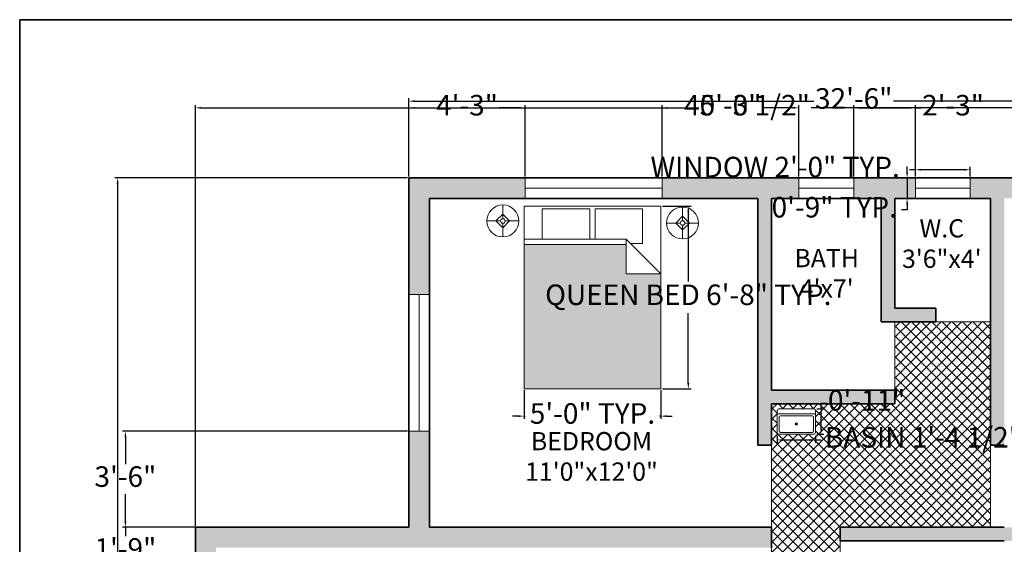
# Model space of a CAD drawing. Units: inches. Extents: x 1329 to 1989, y 1493 to 2072.
# Tile 3 of 4: x 1329 to 1761, y 1842 to 2072. Entities that reach past the tile are written whole.
import ezdxf

# ---------------------------------------------------------------- set-up
doc = ezdxf.new("R2010")
doc.units = ezdxf.units.IN
for name, color, linetype, lineweight in [('A-ANNO-DIMS', 2, 'Continuous', 18), ('A-ANNO-TTLB', 7, 'Continuous', 35), ('A-AREA-IDEN', 7, 'Continuous', 25), ('A-FLOR-FIXT', 8, 'Continuous', 18), ('A-FURN', 8, 'Continuous', 18), ('A-GLAZ', 4, 'Continuous', 18), ('A-WALL', 7, 'Continuous', 35)]:
    doc.layers.add(name, color=color, linetype=linetype, lineweight=lineweight)
for name, color, linetype, lineweight, true_color in [('A-FLOR-PATT', 251, 'Continuous', 13, 0x636466), ('A-FURN-PATT', 18, 'Continuous', 13, 0x000000), ('A-WALL-PATT', 251, 'Continuous', 13, 0x636466)]:
    doc.layers.add(name, color=color, linetype=linetype, lineweight=lineweight, true_color=true_color)
doc.styles.get("Standard").update_dxf_attribs({"font": 'arial.ttf'})
doc.dimstyles.new('ISO-25', dxfattribs={"dimtxt": 9, "dimasz": 2.5, "dimexe": 1.25, "dimexo": 0.625, "dimgap": 2, "dimtad": 0, "dimtih": 1, "dimtoh": 1, "dimdec": 1, "dimlunit": 4, "dimtxsty": 'Standard', "dimcen": 2.5, "dimadec": 0, "dimazin": 0, "dimtfac": 0.5, "dimtdec": 1, "dimtmove": 0, "dimatfit": 3, "dimfxl": 1, "dimarcsym": 0})

# ---------------------------------------------------------------- blocks, each defined once
blk = doc.blocks.new('Bed - Queen')
for p, q in [((0, -80.00003), (0, 0)), ((0, 0), (59.99999, 0)), ((59.99999, 0), (59.99999, -80.00003)), ((7.99999, -1.2), (28.79998, -1.2)), ((7.99999, -14.4), (7.99999, -1.2)), ((28.79998, -1.2), (28.79998, -14.4)), ((31.19999, -1.2), (51.99999, -1.2)), ((31.19999, -14.4), (31.19999, -1.2)), ((51.99999, -1.2), (51.99999, -16.4)), ((0, -14.4), (44.8, -14.4)), ((44.8, -16.8), (0, -16.8)), ((59.99999, -29.6), (44.8, -14.4)), ((44.8, -14.4), (44.8, -29.6)), ((51.99999, -16.4), (46.79936, -16.4)), ((44.8, -29.6), (59.99999, -29.6)), ((59.99999, -80.00003), (0, -80.00003))]:
    blk.add_line(p, q)
blk = doc.blocks.new('Lamp - Table')
for p, q in [((0, 7), (0, 1)), ((-1, 0), (-7, 0)), ((0, 3), (-3, 0)), ((-3, 0), (0, -3)), ((3, 0), (0, 3)), ((0, -3), (3, 0)), ((1, 0), (7, 0)), ((0, -1), (0, -7))]:
    blk.add_line(p, q)
for radius in [7, 1]:
    blk.add_circle((0, 0), radius)
blk = doc.blocks.new('Sink-single - 30 in top')
blk.add_line((-15, -3.999996), (15, -3.999996))
for points in [[(-13.5, 0), (13.5, 0)], [(-15, -18.499996), (-15, -1.5)], [(-13.5, -17.499996), (-13.5, -6.499996)], [(-12.5, -5.499996), (12.5, -5.499996)], [(13.5, -6.499996), (13.5, -17.499996)], [(15, -1.5), (15, -18.499996)], [(13.5, -19.999996), (-13.5, -19.999996)], [(12.5, -18.499996), (-12.5, -18.499996)]]:
    blk.add_lwpolyline(points)
for radius in [1, 0.5]:
    blk.add_circle((0, -11.999996), radius)
for centre, radius, start, end in [((-13.5, -1.5), 1.5, 90, 180), ((-12.5, -6.499996), 1, 90, 180), ((12.5, -6.499996), 1, 0, 90), ((13.5, -1.5), 1.5, 0, 90), ((-13.5, -18.499996), 1.5, 180, 270), ((-12.5, -17.499996), 1, 180, 270), ((12.5, -17.499996), 1, 270, 0), ((13.5, -18.499996), 1.5, 270, 0)]:
    blk.add_arc(centre, radius, start, end)
blk = doc.blocks.new('*D12')
at = {"layer": 'A-ANNO-DIMS', "color": 0, "lineweight": -2, "transparency": 16777216}
for p, q in [((1499.69, 2003.15), (1499.69, 2037.42)), ((1889.69, 2003.15), (1889.69, 2037.42)), ((1502.19, 2036.17), (1677.23, 2036.17)), ((1887.19, 2036.17), (1712.14, 2036.17))]:
    blk.add_line(p, q, dxfattribs=at)
at = {"layer": 'A-ANNO-DIMS', "color": 0, "transparency": 16777216}
for points in [[(1502.19, 2036.58), (1502.19, 2035.75), (1499.69, 2036.17)], [(1887.19, 2036.58), (1887.19, 2035.75), (1889.69, 2036.17)]]:
    blk.add_solid(points, dxfattribs=at)
at = {"layer": 'Defpoints', "color": 0, "transparency": 16777216}
for p in [(1889.69, 2036.17), (1499.69, 2002.52), (1889.69, 2002.52)]:
    blk.add_point(p, dxfattribs=at)
at = {"layer": 'A-ANNO-DIMS', "color": 0, "transparency": 16777216, "insert": (1694.69, 2036.17), "char_height": 9, "attachment_point": 5}
blk.add_mtext('32\'-6"', dxfattribs=at)
blk = doc.blocks.new('*D14')
at = {"layer": 'A-ANNO-DIMS', "color": 0, "lineweight": -2, "transparency": 16777216}
for p, q in [((1499.06, 2002.52), (1370.79, 2002.52)), ((1372.04, 2000.02), (1372.04, 1817.12)), ((1372.04, 1621.02), (1372.04, 1803.93)), ((1499.06, 1618.52), (1370.79, 1618.52))]:
    blk.add_line(p, q, dxfattribs=at)
at = {"layer": 'A-ANNO-DIMS', "color": 0, "transparency": 16777216}
for points in [[(1371.62, 2000.02), (1372.45, 2000.02), (1372.04, 2002.52)], [(1371.62, 1621.02), (1372.45, 1621.02), (1372.04, 1618.52)]]:
    blk.add_solid(points, dxfattribs=at)
at = {"layer": 'Defpoints', "color": 0, "transparency": 16777216}
for p in [(1499.69, 2002.52), (1372.04, 1618.52), (1499.69, 1618.52)]:
    blk.add_point(p, dxfattribs=at)
at = {"layer": 'A-ANNO-DIMS', "color": 0, "transparency": 16777216, "insert": (1372.04, 1810.52), "char_height": 9, "attachment_point": 5}
blk.add_mtext("32'", dxfattribs=at)
blk = doc.blocks.new('WIN-60IN')
for p, q in [((0, 0), (0, 9)), ((60, 0), (60, 9)), ((0, 4.5), (60, 4.5))]:
    blk.add_line(p, q)
blk = doc.blocks.new('WIN-24IN')
for p, q in [((0, 0), (0, 9)), ((24, 0), (24, 9)), ((0, 4.5), (24, 4.5))]:
    blk.add_line(p, q)
blk = doc.blocks.new('*D19')
at = {"layer": 'A-ANNO-DIMS', "color": 0, "lineweight": -2, "transparency": 16777216}
for p, q in [((1721.69, 2003.15), (1721.69, 2007.37)), ((1745.69, 2003.15), (1745.69, 2007.37)), ((1721.69, 2006.12), (1719.19, 2006.12)), ((1743.19, 2006.12), (1724.19, 2006.12))]:
    blk.add_line(p, q, dxfattribs=at)
at = {"layer": 'A-ANNO-DIMS', "color": 0, "transparency": 16777216}
for points in [[(1724.19, 2006.54), (1724.19, 2005.71), (1721.69, 2006.12)], [(1743.19, 2006.54), (1743.19, 2005.71), (1745.69, 2006.12)]]:
    blk.add_solid(points, dxfattribs=at)
at = {"layer": 'Defpoints', "color": 0, "transparency": 16777216}
for p in [(1721.69, 2006.12), (1721.69, 2002.52), (1745.69, 2002.52)]:
    blk.add_point(p, dxfattribs=at)
at = {"layer": 'A-ANNO-DIMS', "color": 0, "transparency": 16777216, "insert": (1660.24, 2006.12), "char_height": 9, "attachment_point": 5}
blk.add_mtext('WINDOW 2\'-0" TYP.', dxfattribs=at)
blk = doc.blocks.new('*D20')
at = {"layer": 'A-ANNO-DIMS', "color": 0, "lineweight": -2, "transparency": 16777216}
for p, q in [((1718.09, 2005.02), (1718.09, 2007.52)), ((1721.06, 2002.52), (1716.84, 2002.52)), ((1718.09, 2002.52), (1718.09, 1993.52)), ((1721.06, 1993.52), (1716.84, 1993.52)), ((1718.09, 1991.02), (1718.09, 1988.52)), ((1718.09, 1988.52), (1715.59, 1988.52))]:
    blk.add_line(p, q, dxfattribs=at)
at = {"layer": 'A-ANNO-DIMS', "color": 0, "transparency": 16777216}
for points in [[(1717.67, 2005.02), (1718.5, 2005.02), (1718.09, 2002.52)], [(1717.67, 1991.02), (1718.5, 1991.02), (1718.09, 1993.52)]]:
    blk.add_solid(points, dxfattribs=at)
at = {"layer": 'Defpoints', "color": 0, "transparency": 16777216}
for p in [(1721.69, 2002.52), (1718.09, 1993.52), (1721.69, 1993.52)]:
    blk.add_point(p, dxfattribs=at)
at = {"layer": 'A-ANNO-DIMS', "color": 0, "transparency": 16777216, "insert": (1686.16, 1988.52), "char_height": 9, "attachment_point": 5}
blk.add_mtext('0\'-9" TYP.', dxfattribs=at)
blk = doc.blocks.new('*D23')
at = {"layer": 'A-ANNO-DIMS', "color": 0, "lineweight": -2, "transparency": 16777216}
for p, q in [((1610.8, 1990.17), (1623.42, 1990.17)), ((1622.17, 1987.67), (1622.17, 1957.1)), ((1622.17, 1912.67), (1622.17, 1943.24)), ((1610.8, 1910.17), (1623.42, 1910.17))]:
    blk.add_line(p, q, dxfattribs=at)
at = {"layer": 'A-ANNO-DIMS', "color": 0, "transparency": 16777216}
for points in [[(1621.76, 1987.67), (1622.59, 1987.67), (1622.17, 1990.17)], [(1621.76, 1912.67), (1622.59, 1912.67), (1622.17, 1910.17)]]:
    blk.add_solid(points, dxfattribs=at)
at = {"layer": 'Defpoints', "color": 0, "transparency": 16777216}
for p in [(1610.17, 1990.17), (1622.17, 1990.17), (1610.17, 1910.17)]:
    blk.add_point(p, dxfattribs=at)
at = {"layer": 'A-ANNO-DIMS', "color": 0, "transparency": 16777216, "insert": (1622.17, 1950.17), "char_height": 9, "attachment_point": 5}
blk.add_mtext('QUEEN BED 6\'-8" TYP.', dxfattribs=at)
blk = doc.blocks.new('*D24')
at = {"layer": 'A-ANNO-DIMS', "color": 0, "lineweight": -2, "transparency": 16777216}
for p, q in [((1550.17, 1909.55), (1550.17, 1896.92)), ((1610.17, 1909.55), (1610.17, 1896.92)), ((1547.67, 1898.17), (1545.17, 1898.17)), ((1550.17, 1898.17), (1550.74, 1898.17)), ((1610.17, 1898.17), (1609.6, 1898.17)), ((1612.67, 1898.17), (1615.17, 1898.17))]:
    blk.add_line(p, q, dxfattribs=at)
at = {"layer": 'A-ANNO-DIMS', "color": 0, "transparency": 16777216}
for points in [[(1547.67, 1898.59), (1547.67, 1897.76), (1550.17, 1898.17)], [(1612.67, 1898.59), (1612.67, 1897.76), (1610.17, 1898.17)]]:
    blk.add_solid(points, dxfattribs=at)
at = {"layer": 'Defpoints', "color": 0, "transparency": 16777216}
for p in [(1550.17, 1910.17), (1610.17, 1910.17), (1610.17, 1898.17)]:
    blk.add_point(p, dxfattribs=at)
at = {"layer": 'A-ANNO-DIMS', "color": 0, "transparency": 16777216, "insert": (1580.17, 1898.17), "char_height": 9, "attachment_point": 5}
blk.add_mtext('5\'-0" TYP.', dxfattribs=at)
blk = doc.blocks.new('*D29')
at = {"layer": 'A-ANNO-DIMS', "color": 0, "lineweight": -2, "transparency": 16777216}
for p, q in [((1661.14, 1889.61), (1661.14, 1886.47)), ((1663.64, 1887.72), (1675.39, 1887.72)), ((1677.89, 1889.61), (1677.89, 1886.47)), ((1677.89, 1887.72), (1680.39, 1887.72))]:
    blk.add_line(p, q, dxfattribs=at)
at = {"layer": 'A-ANNO-DIMS', "color": 0, "transparency": 16777216}
for points in [[(1663.64, 1888.14), (1663.64, 1887.31), (1661.14, 1887.72)], [(1675.39, 1888.14), (1675.39, 1887.31), (1677.89, 1887.72)]]:
    blk.add_solid(points, dxfattribs=at)
at = {"layer": 'Defpoints', "color": 0, "transparency": 16777216}
for p in [(1661.14, 1890.24), (1677.89, 1890.24), (1677.89, 1887.72)]:
    blk.add_point(p, dxfattribs=at)
at = {"layer": 'A-ANNO-DIMS', "color": 0, "transparency": 16777216, "insert": (1725.25, 1887.72), "char_height": 9, "attachment_point": 5}
blk.add_mtext('BASIN 1\'-4 1/2"', dxfattribs=at)
blk = doc.blocks.new('*D30')
at = {"layer": 'A-ANNO-DIMS', "color": 0, "lineweight": -2, "transparency": 16777216}
for p, q in [((1680.4, 1901.4), (1680.4, 1903.9)), ((1680.4, 1903.9), (1682.9, 1903.9)), ((1678.51, 1901.4), (1681.65, 1901.4)), ((1680.4, 1892.74), (1680.4, 1898.9)), ((1678.51, 1890.24), (1681.65, 1890.24))]:
    blk.add_line(p, q, dxfattribs=at)
at = {"layer": 'A-ANNO-DIMS', "color": 0, "transparency": 16777216}
for points in [[(1679.98, 1898.9), (1680.82, 1898.9), (1680.4, 1901.4)], [(1679.98, 1892.74), (1680.82, 1892.74), (1680.4, 1890.24)]]:
    blk.add_solid(points, dxfattribs=at)
at = {"layer": 'Defpoints', "color": 0, "transparency": 16777216}
for p in [(1677.89, 1901.4), (1680.4, 1901.4), (1677.89, 1890.24)]:
    blk.add_point(p, dxfattribs=at)
at = {"layer": 'A-ANNO-DIMS', "color": 0, "transparency": 16777216, "insert": (1700.36, 1903.9), "char_height": 9, "attachment_point": 5}
blk.add_mtext('0\'-11"', dxfattribs=at)
blk = doc.blocks.new('*D37')
at = {"layer": 'A-ANNO-DIMS', "color": 0, "lineweight": -2, "transparency": 16777216}
for p, q in [((1406.14, 1850.15), (1406.14, 2034.47)), ((1408.64, 2033.22), (1619.79, 2033.22)), ((1887.19, 2033.22), (1676.04, 2033.22)), ((1889.69, 2003.15), (1889.69, 2034.47))]:
    blk.add_line(p, q, dxfattribs=at)
at = {"layer": 'A-ANNO-DIMS', "color": 0, "transparency": 16777216}
for points in [[(1408.64, 2033.64), (1408.64, 2032.81), (1406.14, 2033.22)], [(1887.19, 2033.64), (1887.19, 2032.81), (1889.69, 2033.22)]]:
    blk.add_solid(points, dxfattribs=at)
at = {"layer": 'Defpoints', "color": 0, "transparency": 16777216}
for p in [(1889.69, 2033.22), (1889.69, 2002.52), (1406.14, 1849.52)]:
    blk.add_point(p, dxfattribs=at)
at = {"layer": 'A-ANNO-DIMS', "color": 0, "transparency": 16777216, "insert": (1647.91, 2033.22), "char_height": 9, "attachment_point": 5}
blk.add_mtext('40\'-3 1/2"', dxfattribs=at)
blk = doc.blocks.new('*D38')
at = {"layer": 'A-ANNO-DIMS', "color": 0, "lineweight": -2, "transparency": 16777216}
for p, q in [((1890.31, 2002.52), (1921.64, 2002.52)), ((1920.39, 2000.02), (1920.39, 1772.49)), ((1920.39, 1531.65), (1920.39, 1759.18)), ((1759.27, 1529.15), (1921.64, 1529.15))]:
    blk.add_line(p, q, dxfattribs=at)
at = {"layer": 'A-ANNO-DIMS', "color": 0, "transparency": 16777216}
for points in [[(1919.97, 2000.02), (1920.8, 2000.02), (1920.39, 2002.52)], [(1919.97, 1531.65), (1920.8, 1531.65), (1920.39, 1529.15)]]:
    blk.add_solid(points, dxfattribs=at)
at = {"layer": 'Defpoints', "color": 0, "transparency": 16777216}
for p in [(1889.69, 2002.52), (1758.64, 1529.15), (1920.39, 1529.15)]:
    blk.add_point(p, dxfattribs=at)
at = {"layer": 'A-ANNO-DIMS', "color": 0, "transparency": 16777216, "insert": (1920.39, 1765.84), "char_height": 9, "attachment_point": 5}
blk.add_mtext('39\'-5 1/2"', dxfattribs=at)
blk = doc.blocks.new('*D39')
at = {"layer": 'A-ANNO-DIMS', "color": 0, "lineweight": -2, "transparency": 16777216}
for p, q in [((1499.69, 2003.15), (1499.69, 2034.47)), ((1502.19, 2033.22), (1511.04, 2033.22)), ((1548.19, 2033.22), (1539.33, 2033.22)), ((1550.69, 2003.15), (1550.69, 2034.47))]:
    blk.add_line(p, q, dxfattribs=at)
at = {"layer": 'A-ANNO-DIMS', "color": 0, "transparency": 16777216}
for points in [[(1502.19, 2033.64), (1502.19, 2032.81), (1499.69, 2033.22)], [(1548.19, 2033.64), (1548.19, 2032.81), (1550.69, 2033.22)]]:
    blk.add_solid(points, dxfattribs=at)
at = {"layer": 'Defpoints', "color": 0, "transparency": 16777216}
for p in [(1550.69, 2033.22), (1499.69, 2002.52), (1550.69, 2002.52)]:
    blk.add_point(p, dxfattribs=at)
at = {"layer": 'A-ANNO-DIMS', "color": 0, "transparency": 16777216, "insert": (1525.19, 2033.22), "char_height": 9, "attachment_point": 5}
blk.add_mtext('4\'-3"', dxfattribs=at)
blk = doc.blocks.new('*D40')
at = {"layer": 'A-ANNO-DIMS', "color": 0, "lineweight": -2, "transparency": 16777216}
for p, q in [((1610.69, 2003.15), (1610.69, 2034.47)), ((1613.19, 2033.22), (1626.72, 2033.22)), ((1668.19, 2033.22), (1654.65, 2033.22)), ((1670.69, 2003.15), (1670.69, 2034.47))]:
    blk.add_line(p, q, dxfattribs=at)
at = {"layer": 'A-ANNO-DIMS', "color": 0, "transparency": 16777216}
for points in [[(1613.19, 2033.64), (1613.19, 2032.81), (1610.69, 2033.22)], [(1668.19, 2033.64), (1668.19, 2032.81), (1670.69, 2033.22)]]:
    blk.add_solid(points, dxfattribs=at)
at = {"layer": 'Defpoints', "color": 0, "transparency": 16777216}
for p in [(1670.69, 2033.22), (1610.69, 2002.52), (1670.69, 2002.52)]:
    blk.add_point(p, dxfattribs=at)
at = {"layer": 'A-ANNO-DIMS', "color": 0, "transparency": 16777216, "insert": (1640.69, 2033.22), "char_height": 9, "attachment_point": 5}
blk.add_mtext('5\'-0"', dxfattribs=at)
blk = doc.blocks.new('*D41')
at = {"layer": 'A-ANNO-DIMS', "color": 0, "lineweight": -2, "transparency": 16777216}
for p, q in [((1694.69, 2003.15), (1694.69, 2034.47)), ((1697.19, 2033.22), (1719.19, 2033.22)), ((1721.69, 2003.15), (1721.69, 2034.47)), ((1721.69, 2033.22), (1724.19, 2033.22))]:
    blk.add_line(p, q, dxfattribs=at)
at = {"layer": 'A-ANNO-DIMS', "color": 0, "transparency": 16777216}
for points in [[(1697.19, 2033.64), (1697.19, 2032.81), (1694.69, 2033.22)], [(1719.19, 2033.64), (1719.19, 2032.81), (1721.69, 2033.22)]]:
    blk.add_solid(points, dxfattribs=at)
at = {"layer": 'Defpoints', "color": 0, "transparency": 16777216}
for p in [(1721.69, 2033.22), (1694.69, 2002.52), (1721.69, 2002.52)]:
    blk.add_point(p, dxfattribs=at)
at = {"layer": 'A-ANNO-DIMS', "color": 0, "transparency": 16777216, "insert": (1738.23, 2033.22), "char_height": 9, "attachment_point": 5}
blk.add_mtext('2\'-3"', dxfattribs=at)
blk = doc.blocks.new('*D45')
at = {"layer": 'A-ANNO-DIMS', "color": 0, "lineweight": -2, "transparency": 16777216}
for p, q in [((1499.06, 1891.52), (1374.19, 1891.52)), ((1375.44, 1889.02), (1375.44, 1877.12)), ((1375.44, 1852.02), (1375.44, 1863.93)), ((1499.06, 1849.52), (1374.19, 1849.52))]:
    blk.add_line(p, q, dxfattribs=at)
at = {"layer": 'A-ANNO-DIMS', "color": 0, "transparency": 16777216}
for points in [[(1375.02, 1889.02), (1375.86, 1889.02), (1375.44, 1891.52)], [(1375.02, 1852.02), (1375.86, 1852.02), (1375.44, 1849.52)]]:
    blk.add_solid(points, dxfattribs=at)
at = {"layer": 'Defpoints', "color": 0, "transparency": 16777216}
for p in [(1375.44, 1891.52), (1499.69, 1891.52), (1499.69, 1849.52)]:
    blk.add_point(p, dxfattribs=at)
at = {"layer": 'A-ANNO-DIMS', "color": 0, "transparency": 16777216, "insert": (1375.44, 1870.52), "char_height": 9, "attachment_point": 5}
blk.add_mtext('3\'-6"', dxfattribs=at)
blk = doc.blocks.new('*D47')
at = {"layer": 'A-ANNO-DIMS', "color": 0, "lineweight": -2, "transparency": 16777216}
for p, q in [((1375.44, 1852.02), (1375.44, 1854.52)), ((1405.52, 1849.52), (1374.19, 1849.52)), ((1375.44, 1849.52), (1375.44, 1845.62)), ((1375.44, 1828.52), (1375.44, 1832.43)), ((1405.52, 1828.52), (1374.19, 1828.52)), ((1375.44, 1826.02), (1375.44, 1823.52))]:
    blk.add_line(p, q, dxfattribs=at)
at = {"layer": 'A-ANNO-DIMS', "color": 0, "transparency": 16777216}
for points in [[(1375.02, 1852.02), (1375.86, 1852.02), (1375.44, 1849.52)], [(1375.02, 1826.02), (1375.86, 1826.02), (1375.44, 1828.52)]]:
    blk.add_solid(points, dxfattribs=at)
at = {"layer": 'Defpoints', "color": 0, "transparency": 16777216}
for p in [(1406.14, 1849.52), (1375.44, 1828.52), (1406.14, 1828.52)]:
    blk.add_point(p, dxfattribs=at)
at = {"layer": 'A-ANNO-DIMS', "color": 0, "transparency": 16777216, "insert": (1375.44, 1839.02), "char_height": 9, "attachment_point": 5}
blk.add_mtext('1\'-9"', dxfattribs=at)

msp = doc.modelspace()

# ---------------------------------------------------------------- hatches: boundary and pattern name
at = {"layer": 'A-FLOR-PATT'}
h = msp.add_hatch(dxfattribs=at)
h.set_pattern_fill('ANSI37', color=256)
h.paths.add_polyline_path([(1754.69, 1885.52), (1754.69, 1939.52), (1730.69, 1939.52), (1712.69, 1939.52), (1712.69, 1909.52), (1712.69, 1903.52), (1706.69, 1903.52), (1658.69, 1903.52), (1658.69, 1885.52), (1658.69, 1804.52), (1658.69, 1759.52), (1688.69, 1759.52), (1688.69, 1795.52), (1688.69, 1843.52), (1688.69, 1849.52), (1754.69, 1849.52)])
h.paths.add_polyline_path([(1677.05, 1890.24), (1661.98, 1890.24, -0.414214), (1661.14, 1891.07), (1661.14, 1900.56, -0.414214), (1661.98, 1901.4), (1677.05, 1901.4, -0.414214), (1677.89, 1900.56), (1677.89, 1891.07, -0.414214)], flags=16)
h.paths.add_polyline_path([(1676.49, 1891.07), (1662.54, 1891.07, -0.414214), (1661.98, 1891.63), (1661.98, 1897.77, -0.414214), (1662.54, 1898.33), (1676.49, 1898.33, -0.414214), (1677.05, 1897.77), (1677.05, 1891.63, -0.414214)], flags=0)
h.paths.add_polyline_path([(1668.96, 1894.7, -1), (1670.07, 1894.7, -1)], flags=0)
h.paths.add_polyline_path([(1669.23, 1894.7, -1), (1669.79, 1894.7, -1)], flags=0)
at = {"layer": 'A-FURN-PATT'}
h = msp.add_hatch(color=256, dxfattribs=at)
h.dxf.hatch_style = 1
h.paths.add_polyline_path([(1610.17, 1960.57), (1594.97, 1960.57), (1594.97, 1973.37), (1550.17, 1973.37), (1550.17, 1910.17), (1610.17, 1910.17)])
h.paths.add_polyline_path([(1850.61, 1961.54), (1835.41, 1961.54), (1835.41, 1974.34), (1790.61, 1974.34), (1790.61, 1911.14), (1850.61, 1911.14)])
at = {"layer": 'A-WALL-PATT'}
h = msp.add_hatch(color=256, dxfattribs=at)
h.dxf.hatch_style = 1
h.paths.add_polyline_path([(1550.69, 2002.52), (1499.69, 2002.52), (1499.69, 1951.52), (1508.69, 1951.52), (1508.69, 1993.52), (1550.69, 1993.52)])
h.paths.add_polyline_path([(1670.69, 2002.52), (1610.69, 2002.52), (1610.69, 1993.52), (1652.69, 1993.52), (1652.69, 1885.52), (1658.69, 1885.52), (1658.69, 1903.52), (1706.69, 1903.52), (1712.69, 1903.52), (1712.69, 1909.52), (1706.69, 1909.52), (1658.69, 1909.52), (1658.69, 1993.52), (1670.69, 1993.52)])
h.paths.add_polyline_path([(1721.69, 2002.52), (1694.69, 2002.52), (1694.69, 1993.52), (1706.69, 1993.52), (1706.69, 1939.52), (1712.69, 1939.52), (1730.69, 1939.52), (1730.69, 1945.52), (1712.69, 1945.52), (1712.69, 1993.52), (1721.69, 1993.52)])
h.paths.add_polyline_path([(1790.69, 2002.52), (1745.69, 2002.52), (1745.69, 1993.52), (1754.69, 1993.52), (1754.69, 1945.52), (1754.69, 1939.52), (1754.69, 1885.52), (1760.69, 1885.52), (1760.69, 1993.52), (1790.69, 1993.52)])
h.paths.add_polyline_path([(1889.69, 2002.52), (1850.69, 2002.52), (1850.69, 1993.52), (1880.69, 1993.52), (1880.69, 1951.52), (1889.69, 1951.52)])
h.paths.add_polyline_path([(1889.69, 1891.52), (1880.69, 1891.52), (1880.69, 1849.52), (1760.69, 1849.52), (1754.69, 1849.52), (1688.69, 1849.52), (1688.69, 1843.52), (1697.69, 1843.52), (1760.69, 1843.52), (1880.69, 1843.52), (1880.69, 1798.52), (1889.69, 1798.52)])
h.paths.add_polyline_path([(1658.69, 1849.52), (1652.69, 1849.52), (1508.69, 1849.52), (1508.69, 1891.52), (1499.69, 1891.52), (1499.69, 1849.52), (1406.14, 1849.52), (1406.14, 1828.52), (1415.14, 1828.52), (1415.14, 1840.52), (1508.69, 1840.52), (1652.69, 1840.52), (1658.69, 1840.52)])
h.paths.add_polyline_path([(1658.69, 1804.52), (1652.69, 1804.52), (1652.69, 1768.52), (1508.69, 1768.52), (1415.14, 1768.52), (1415.14, 1780.52), (1406.14, 1780.52), (1406.14, 1759.52), (1499.69, 1759.52), (1499.69, 1709.88), (1508.69, 1709.88), (1508.69, 1759.52), (1658.69, 1759.52)])
h.paths.add_polyline_path([(1508.69, 1649.88), (1499.69, 1649.88), (1499.69, 1618.52), (1568.69, 1618.52), (1568.69, 1627.52), (1508.69, 1627.52)])
h.paths.add_polyline_path([(1697.69, 1684.52), (1697.69, 1693.52), (1697.69, 1795.52), (1688.69, 1795.52), (1688.69, 1693.52), (1688.69, 1684.52), (1688.69, 1627.52), (1628.69, 1627.52), (1628.69, 1618.52), (1688.69, 1618.52), (1688.69, 1588.52), (1697.69, 1588.52), (1697.69, 1618.52)])
h.paths.add_polyline_path([(1790.69, 1693.52), (1760.69, 1693.52), (1745.69, 1693.52), (1745.69, 1684.52), (1760.69, 1684.52), (1790.69, 1684.52)])
h.paths.add_polyline_path([(1889.69, 1738.52), (1880.69, 1738.52), (1880.69, 1693.52), (1850.69, 1693.52), (1850.69, 1684.52), (1880.69, 1684.52), (1889.69, 1684.52)])

# ---------------------------------------------------------------- linework, layer by layer
at = {"layer": 'A-ANNO-TTLB'}
msp.add_lwpolyline([(1329.11, 2071.84), (1964.17, 2071.84), (1964.17, 1500.65), (1329.11, 1500.65)], close=True, dxfattribs=at)
at = {"layer": 'A-FLOR-PATT'}
for p, q in [((1712.69, 1909.52), (1712.69, 1939.52)), ((1730.69, 1939.52), (1754.69, 1939.52)), ((1658.69, 1804.52), (1658.69, 1885.52)), ((1754.69, 1885.52), (1754.69, 1849.52)), ((1688.69, 1843.52), (1688.69, 1795.52))]:
    msp.add_line(p, q, dxfattribs=at)
at = {"layer": 'A-WALL'}
for p, q in [((1499.69, 2002.52), (1889.69, 2002.52)), ((1499.69, 2002.52), (1499.69, 1849.52)), ((1508.69, 1993.52), (1652.69, 1993.52)), ((1508.69, 1993.52), (1508.69, 1849.52)), ((1652.69, 1993.52), (1652.69, 1885.52)), ((1658.69, 1993.52), (1658.69, 1909.52)), ((1658.69, 1993.52), (1706.69, 1993.52)), ((1706.69, 1993.52), (1706.69, 1939.52)), ((1712.69, 1993.52), (1712.69, 1945.52)), ((1712.69, 1993.52), (1754.69, 1993.52)), ((1754.69, 1993.52), (1754.69, 1945.52)), ((1712.69, 1945.52), (1730.69, 1945.52)), ((1730.69, 1945.52), (1730.69, 1939.52)), ((1754.69, 1945.52), (1754.69, 1939.52)), ((1712.69, 1939.52), (1706.69, 1939.52)), ((1712.69, 1939.52), (1730.69, 1939.52)), ((1754.69, 1939.52), (1754.69, 1885.52)), ((1658.69, 1909.52), (1706.69, 1909.52)), ((1706.69, 1909.52), (1712.69, 1909.52)), ((1712.69, 1909.52), (1712.69, 1903.52)), ((1658.69, 1903.52), (1706.69, 1903.52)), ((1658.69, 1903.52), (1658.69, 1885.52)), ((1706.69, 1903.52), (1712.69, 1903.52)), ((1652.69, 1885.52), (1658.69, 1885.52)), ((1754.69, 1885.52), (1760.69, 1885.52)), ((1406.14, 1759.52), (1406.14, 1849.52)), ((1499.69, 1849.52), (1406.14, 1849.52)), ((1508.69, 1849.52), (1652.69, 1849.52)), ((1652.69, 1849.52), (1658.69, 1849.52)), ((1658.69, 1849.52), (1658.69, 1840.52)), ((1754.69, 1849.52), (1688.69, 1849.52)), ((1688.69, 1849.52), (1688.69, 1843.52)), ((1688.69, 1843.52), (1688.69, 1849.52)), ((1754.69, 1849.52), (1760.69, 1849.52)), ((1697.69, 1843.52), (1688.69, 1843.52)), ((1760.69, 1843.52), (1697.69, 1843.52))]:
    msp.add_line(p, q, dxfattribs=at)

# ---------------------------------------------------------------- block references
at = {"layer": 'A-FLOR-FIXT', "xscale": 0.5582271038075876, "yscale": 0.5582271038075876, "zscale": 0.5582271038075876}
msp.add_blockref('Sink-single - 30 in top', (1669.51, 1901.4), dxfattribs=at)
at = {"layer": 'A-FURN'}
for name, p in [('Lamp - Table', (1540.86, 1983.67)), ('Bed - Queen', (1550.17, 1990.17)), ('Lamp - Table', (1619.66, 1982.78))]:
    msp.add_blockref(name, p, dxfattribs=at)
at = {"layer": 'A-GLAZ'}
for name, p, rotation in [('WIN-60IN', (1610.69, 2002.52), 180), ('WIN-24IN', (1745.69, 2002.52), 180), ('WIN-60IN', (1499.69, 1951.52), 269.9999999999998)]:
    msp.add_blockref(name, p, dxfattribs=dict(at, rotation=rotation))
msp.add_blockref('WIN-24IN', (1670.69, 1993.52), dxfattribs=at)

# ---------------------------------------------------------------- texts
at = {"layer": 'A-AREA-IDEN', "char_height": 8, "attachment_point": 1}
for s, width, insert in [('\\pxqc;{\\fArial|b1|i0|c0|p34;W.C\\P3\'6"x4\'}', 35.6826, (1715.43, 1984.45)), ("\\pxqc;{\\fArial|b1|i0|c0|p34;BATH\\P4'x7'}", 41.0434, (1662.32, 1971.4)), ('\\pxqc;{\\fArial|b1|i0|c0|p34;BEDROOM\\P11\'0"x12\'0}"', 108.1077, (1525.67, 1891.2))]:
    msp.add_mtext_dynamic_manual_height_columns(s, width=width, gutter_width=12.5, heights=[0], dxfattribs=dict(at, insert=insert))

# ---------------------------------------------------------------- dimensions: what is measured, and where the dimension line sits
at = {"layer": 'A-ANNO-DIMS'}
for base, p1, p2, override, picture, middle in [((1889.6864, 2033.2237), (1406.141, 1849.5237), (1889.6864, 2002.5237), {"dimdec": 1, "dimlfac": 1, "dimrnd": 0, "dimzin": 1, "dimdsep": 46, "dimlunit": 4, "dimfrac": 2}, '*D37', (1647.9137, 2033.2237)), ((1889.69, 2036.17), (1499.69, 2002.52), (1889.69, 2002.52), {"dimclrd": 0, "dimclre": 0, "dimclrt": 0}, '*D12', (1694.69, 2036.17)), ((1550.69, 2033.22), (1499.69, 2002.52), (1550.69, 2002.52), {"dimdec": 1, "dimlfac": 1, "dimrnd": 0, "dimzin": 1, "dimdsep": 46, "dimlunit": 4, "dimfrac": 2}, '*D39', (1525.19, 2033.22)), ((1670.69, 2033.22), (1610.69, 2002.52), (1670.69, 2002.52), {"dimdec": 1, "dimlfac": 1, "dimrnd": 0, "dimzin": 1, "dimdsep": 46, "dimlunit": 4, "dimfrac": 2}, '*D40', (1640.69, 2033.22)), ((1721.69, 2033.22), (1694.69, 2002.52), (1721.69, 2002.52), {"dimdec": 1, "dimlfac": 1, "dimrnd": 0, "dimzin": 1, "dimdsep": 46, "dimlunit": 4, "dimfrac": 2}, '*D41', (1738.23, 2033.22))]:
    dim = msp.add_linear_dim(base=base, p1=p1, p2=p2, dimstyle='ISO-25', override=override, dxfattribs=at)
    dim.commit()
    dim.dimension.update_dxf_attribs({"geometry": picture, "text_midpoint": middle})
for base, p1, p2, angle, text, picture, middle in [((1721.69, 2006.12), (1745.69, 2002.52), (1721.69, 2002.52), 180, 'WINDOW <> TYP.', '*D19', (1660.24, 2006.12)), ((1718.09, 1993.52), (1721.69, 2002.52), (1721.69, 1993.52), 270, '<> TYP.', '*D20', (1686.16, 1988.52)), ((1622.17, 1990.17), (1610.17, 1910.17), (1610.17, 1990.17), 90, 'QUEEN BED <> TYP.', '*D23', (1622.17, 1950.17))]:
    dim = msp.add_linear_dim(base=base, p1=p1, p2=p2, angle=angle, text=text, dimstyle='ISO-25', override={"dimdec": 1, "dimlfac": 1, "dimrnd": 0, "dimzin": 1, "dimdsep": 46, "dimlunit": 4, "dimfrac": 2}, dxfattribs=at)
    dim.commit()
    dim.dimension.update_dxf_attribs({"geometry": picture, "text_midpoint": middle})
for base, p1, p2, override, picture, middle in [((1372.04, 1618.52), (1499.69, 2002.52), (1499.69, 1618.52), {"dimclrd": 0, "dimclre": 0, "dimclrt": 0}, '*D14', (1372.04, 1810.52)), ((1920.39, 1529.15), (1889.69, 2002.52), (1758.64, 1529.15), {"dimdec": 1, "dimlfac": 1, "dimrnd": 0, "dimzin": 1, "dimdsep": 46, "dimlunit": 4, "dimfrac": 2}, '*D38', (1920.39, 1765.84)), ((1680.4, 1901.4), (1677.89, 1890.24), (1677.89, 1901.4), {"dimdec": 1, "dimlfac": 1, "dimrnd": 0, "dimzin": 1, "dimdsep": 46, "dimlunit": 4, "dimfrac": 2}, '*D30', (1700.36, 1903.9)), ((1375.44, 1891.52), (1499.69, 1849.52), (1499.69, 1891.52), {"dimdec": 1, "dimlfac": 1, "dimrnd": 0, "dimzin": 1, "dimdsep": 46, "dimlunit": 4, "dimfrac": 2}, '*D45', (1375.44, 1870.52)), ((1375.44, 1828.52), (1406.14, 1849.52), (1406.14, 1828.52), {"dimdec": 1, "dimlfac": 1, "dimrnd": 0, "dimzin": 1, "dimdsep": 46, "dimlunit": 4, "dimfrac": 2}, '*D47', (1375.44, 1839.02))]:
    dim = msp.add_linear_dim(base=base, p1=p1, p2=p2, angle=90, dimstyle='ISO-25', override=override, dxfattribs=at)
    dim.commit()
    dim.dimension.update_dxf_attribs({"geometry": picture, "text_midpoint": middle})
for base, p1, p2, text, picture, middle in [((1610.17, 1898.17), (1550.17, 1910.17), (1610.17, 1910.17), '<> TYP.', '*D24', (1580.17, 1898.17)), ((1677.8867, 1887.7233), (1661.1398, 1890.2354), (1677.8867, 1890.2354), 'BASIN <>', '*D29', (1725.2472, 1887.7233))]:
    dim = msp.add_linear_dim(base=base, p1=p1, p2=p2, text=text, dimstyle='ISO-25', override={"dimdec": 1, "dimlfac": 1, "dimrnd": 0, "dimzin": 1, "dimdsep": 46, "dimlunit": 4, "dimfrac": 2}, dxfattribs=at)
    dim.commit()
    dim.dimension.update_dxf_attribs({"geometry": picture, "text_midpoint": middle})

doc.saveas('drawing.dxf')
